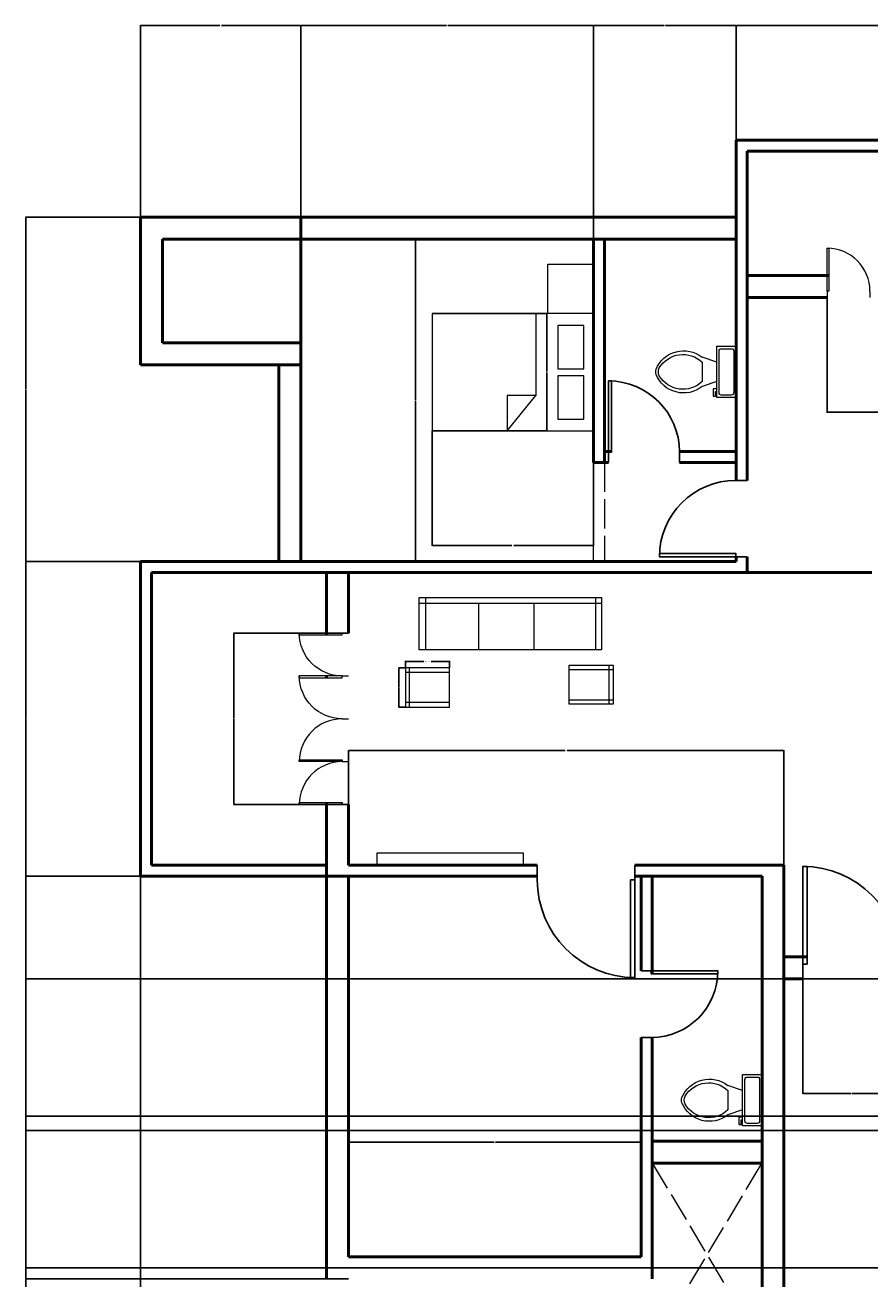
# Model space of a CAD drawing. Units: inches. Extents: x 2032 to 3981, y 840 to 2177.
# Tile 4 of 6: x 2032 to 2378, y 1354 to 1868. Entities that reach past the tile are written whole.
import ezdxf

# ---------------------------------------------------------------- set-up
doc = ezdxf.new("R2010")
doc.units = ezdxf.units.IN
doc.linetypes.add('ACAD_ISO02W100', pattern=[15, 12, -3])
for name, color, linetype, lineweight in [('A-ANNO-DIMS', 2, 'Continuous', 18), ('A-DOOR', 3, 'Continuous', 25), ('A-FLOR-FIXT', 9, 'Continuous', 18), ('A-FLOR-OPEN', 8, 'ACAD_ISO02W100', 13), ('A-FURN', 8, 'Continuous', 18), ('A-GLAZ', 4, 'Continuous', 18), ('A-WALL', 7, 'Continuous', 50), ('A-WALL-OVHD', 8, 'ACAD_ISO02W100', 18)]:
    doc.layers.add(name, color=color, linetype=linetype, lineweight=lineweight)
doc.styles.get("Standard").update_dxf_attribs({"font": 'arial.ttf'})
doc.dimstyles.get("Standard").update_dxf_attribs({"dimtxt": 0.18, "dimasz": 0.18, "dimexe": 0.18, "dimexo": 0.0625, "dimgap": 0.09, "dimtad": 0, "dimtih": 1, "dimtoh": 1, "dimdec": 4, "dimzin": 0, "dimdsep": 46, "dimtxsty": 'Standard', "dimcen": 0.09, "dimadec": 0, "dimazin": 0, "dimtfac": 1, "dimtdec": 4, "dimtofl": 0, "dimtmove": 0, "dimatfit": 3, "dimfxl": 1, "dimtolj": 1, "dimtzin": 0, "dimarcsym": 0})

# ---------------------------------------------------------------- blocks, each defined once
blk = doc.blocks.new('*U2')
for p, q in [((0, 0), (0, -6)), ((40, 0), (40, -6))]:
    blk.add_line(p, q)
blk.add_lwpolyline([(0, 0), (0, 40), (1.75, 40), (1.75, 0)], close=True)
blk.add_arc((0, 0), 40, 0, 90)
blk = doc.blocks.new('*U4')
for p, q in [((9.5, -6), (9.5, -2)), ((-10, -8.5), (-8, -8.5)), ((-10, -9.5), (-10, -8.5)), ((-7, -9.5), (-10, -9.5)), ((-8, -8.5), (-8, -8)), ((-7, -8), (-7, -9.5)), ((-4, -8), (-6, -14)), ((4, -8), (6, -14)), ((4, -14), (-4, -14))]:
    blk.add_line(p, q)
blk.add_lwpolyline([(10.5, -8), (10.5, 0), (-10.5, 0), (-10.5, -8)], close=True)
for points in [[(-9.5, -2), (-9.5, -6)], [(8.5, -1), (-8.5, -1)], [(-8.5, -7), (8.5, -7)]]:
    blk.add_lwpolyline(points)
for centre, radius, start, end in [((-8.62, -1.88), 0.884, 81.8699, 188.1301), ((8.62, -1.88), 0.884, 351.8699, 98.1301), ((-8.62, -6.12), 0.884, 171.8699, 278.1301), ((8.62, -6.12), 0.884, 261.8699, 8.1301), ((3.52, -21.58), 12.17, 141.4691, 247.9714), ((4.2, -21.82), 11.33, 136.3677, 238.9468), ((-3.52, -21.58), 12.17, 292.0284, 38.5307), ((-4.2, -21.82), 11.33, 301.053, 43.6321), ((0, -27.88), 4, 245.7318, 294.2682), ((0, -29), 4, 254.8605, 285.1395)]:
    blk.add_arc(centre, radius, start, end)
blk = doc.blocks.new('CHAIR-LOUNGE')
for p, q in [((1.71, 0), (1.71, 16.03)), ((18.07, 14.22), (0, 14.22)), ((18.07, 1.82), (0, 1.82))]:
    blk.add_line(p, q)
blk.add_lwpolyline([(18.07, 16.03), (0, 16.03), (0, 0), (18.07, 0)], close=True)
blk = doc.blocks.new('*D10')
at = {"layer": 'A-ANNO-DIMS', "color": 0, "lineweight": -2, "transparency": 16777216}
for p, q in [((2187.53, 1604.35), (2187.53, 1607.17)), ((2187.71, 1606.99), (2195.05, 1606.99)), ((2205.43, 1606.99), (2198.09, 1606.99)), ((2205.61, 1604.35), (2205.61, 1607.17))]:
    blk.add_line(p, q, dxfattribs=at)
at = {"layer": 'A-ANNO-DIMS', "color": 0, "lineweight": 100, "transparency": 16777216}
for points in [[(2187.71, 1607.02), (2187.71, 1606.96), (2187.53, 1606.99)], [(2205.43, 1607.02), (2205.43, 1606.96), (2205.61, 1606.99)]]:
    blk.add_solid(points, dxfattribs=at)
at = {"layer": 'Defpoints', "color": 0, "lineweight": 100, "transparency": 16777216}
for p in [(2187.53, 1604.28), (2205.61, 1606.99), (2205.61, 1604.28)]:
    blk.add_point(p, dxfattribs=at)
at = {"layer": 'A-ANNO-DIMS', "color": 0, "transparency": 16777216, "insert": (2196.57, 1606.99), "char_height": 0.18, "attachment_point": 5}
blk.add_mtext('\\A1;LOUNGE CHAIR 18 TYP.', dxfattribs=at)
blk = doc.blocks.new('*D11')
at = {"layer": 'A-ANNO-DIMS', "color": 0, "lineweight": -2, "transparency": 16777216}
for p, q in [((2187.47, 1604.28), (2184.64, 1604.28)), ((2184.82, 1604.1), (2184.82, 1596.45)), ((2184.82, 1588.43), (2184.82, 1596.09)), ((2187.47, 1588.25), (2184.64, 1588.25))]:
    blk.add_line(p, q, dxfattribs=at)
at = {"layer": 'A-ANNO-DIMS', "color": 0, "lineweight": 100, "transparency": 16777216}
for points in [[(2184.79, 1604.1), (2184.85, 1604.1), (2184.82, 1604.28)], [(2184.79, 1588.43), (2184.85, 1588.43), (2184.82, 1588.25)]]:
    blk.add_solid(points, dxfattribs=at)
at = {"layer": 'Defpoints', "color": 0, "lineweight": 100, "transparency": 16777216}
for p in [(2184.82, 1604.28), (2187.53, 1604.28), (2187.53, 1588.25)]:
    blk.add_point(p, dxfattribs=at)
at = {"layer": 'A-ANNO-DIMS', "color": 0, "transparency": 16777216, "insert": (2184.82, 1596.27), "char_height": 0.18, "attachment_point": 5}
blk.add_mtext('\\A1;16 TYP.', dxfattribs=at)
blk = doc.blocks.new('*D14')
at = {"layer": 'A-ANNO-DIMS', "color": 0, "lineweight": -2, "transparency": 16777216}
for p, q in [((2078.89, 1518.9), (2078.89, 840.08)), ((2677.35, 1476.9), (2677.35, 840.08)), ((2079.07, 840.26), (2377.73, 840.26)), ((2677.17, 840.26), (2378.52, 840.26))]:
    blk.add_line(p, q, dxfattribs=at)
at = {"layer": 'A-ANNO-DIMS', "color": 0, "lineweight": 100, "transparency": 16777216}
for points in [[(2079.07, 840.29), (2079.07, 840.23), (2078.89, 840.26)], [(2677.17, 840.29), (2677.17, 840.23), (2677.35, 840.26)]]:
    blk.add_solid(points, dxfattribs=at)
at = {"layer": 'Defpoints', "color": 0, "lineweight": 100, "transparency": 16777216}
for p in [(2078.89, 1518.96), (2677.35, 1476.96), (2677.35, 840.26)]:
    blk.add_point(p, dxfattribs=at)
at = {"layer": 'A-ANNO-DIMS', "color": 0, "transparency": 16777216, "insert": (2378.12, 840.26), "char_height": 0.18, "attachment_point": 5}
blk.add_mtext('\\A1;598.5', dxfattribs=at)
blk = doc.blocks.new('*D16')
at = {"layer": 'A-ANNO-DIMS', "color": 0, "lineweight": -2, "transparency": 16777216}
for p, q in [((2078.89, 1789.02), (2078.89, 1867.7)), ((2079.07, 1867.52), (2111.37, 1867.52)), ((2144.45, 1867.52), (2112.15, 1867.52)), ((2144.63, 1789.02), (2144.63, 1867.7))]:
    blk.add_line(p, q, dxfattribs=at)
at = {"layer": 'A-ANNO-DIMS', "color": 0, "lineweight": 100, "transparency": 16777216}
for points in [[(2079.07, 1867.55), (2079.07, 1867.49), (2078.89, 1867.52)], [(2144.45, 1867.55), (2144.45, 1867.49), (2144.63, 1867.52)]]:
    blk.add_solid(points, dxfattribs=at)
at = {"layer": 'Defpoints', "color": 0, "lineweight": 100, "transparency": 16777216}
for p in [(2144.63, 1867.52), (2078.89, 1788.96), (2144.63, 1788.96)]:
    blk.add_point(p, dxfattribs=at)
at = {"layer": 'A-ANNO-DIMS', "color": 0, "transparency": 16777216, "insert": (2111.76, 1867.52), "char_height": 0.18, "attachment_point": 5}
blk.add_mtext('\\A1;65.74', dxfattribs=at)
blk = doc.blocks.new('*D17')
at = {"layer": 'A-ANNO-DIMS', "color": 0, "lineweight": -2, "transparency": 16777216}
for p, q in [((2144.63, 1789.02), (2144.63, 1867.7)), ((2144.81, 1867.52), (2204.35, 1867.52)), ((2264.45, 1867.52), (2204.91, 1867.52)), ((2264.63, 1780.02), (2264.63, 1867.7))]:
    blk.add_line(p, q, dxfattribs=at)
at = {"layer": 'A-ANNO-DIMS', "color": 0, "lineweight": 100, "transparency": 16777216}
for points in [[(2144.81, 1867.55), (2144.81, 1867.49), (2144.63, 1867.52)], [(2264.45, 1867.55), (2264.45, 1867.49), (2264.63, 1867.52)]]:
    blk.add_solid(points, dxfattribs=at)
at = {"layer": 'Defpoints', "color": 0, "lineweight": 100, "transparency": 16777216}
for p in [(2264.63, 1867.52), (2144.63, 1788.96), (2264.63, 1779.96)]:
    blk.add_point(p, dxfattribs=at)
at = {"layer": 'A-ANNO-DIMS', "color": 0, "transparency": 16777216, "insert": (2204.63, 1867.52), "char_height": 0.18, "attachment_point": 5}
blk.add_mtext('\\A1;120', dxfattribs=at)
blk = doc.blocks.new('*D18')
at = {"layer": 'A-ANNO-DIMS', "color": 0, "lineweight": -2, "transparency": 16777216}
for p, q in [((2264.63, 1780.02), (2264.63, 1867.7)), ((2264.81, 1867.52), (2293.55, 1867.52)), ((2322.95, 1867.52), (2294.2, 1867.52)), ((2323.13, 1820.58), (2323.13, 1867.7))]:
    blk.add_line(p, q, dxfattribs=at)
at = {"layer": 'A-ANNO-DIMS', "color": 0, "lineweight": 100, "transparency": 16777216}
for points in [[(2264.81, 1867.55), (2264.81, 1867.49), (2264.63, 1867.52)], [(2322.95, 1867.55), (2322.95, 1867.49), (2323.13, 1867.52)]]:
    blk.add_solid(points, dxfattribs=at)
at = {"layer": 'Defpoints', "color": 0, "lineweight": 100, "transparency": 16777216}
for p in [(2323.13, 1867.52), (2323.13, 1820.52), (2264.63, 1779.96)]:
    blk.add_point(p, dxfattribs=at)
at = {"layer": 'A-ANNO-DIMS', "color": 0, "transparency": 16777216, "insert": (2293.88, 1867.52), "char_height": 0.18, "attachment_point": 5}
blk.add_mtext('\\A1;58.5', dxfattribs=at)
blk = doc.blocks.new('*D19')
at = {"layer": 'A-ANNO-DIMS', "color": 0, "lineweight": -2, "transparency": 16777216}
for p, q in [((2323.13, 1820.58), (2323.13, 1867.7)), ((2323.31, 1867.52), (2389.49, 1867.52)), ((2456.45, 1867.52), (2390.26, 1867.52)), ((2456.63, 1820.58), (2456.63, 1867.7))]:
    blk.add_line(p, q, dxfattribs=at)
at = {"layer": 'A-ANNO-DIMS', "color": 0, "lineweight": 100, "transparency": 16777216}
for points in [[(2323.31, 1867.55), (2323.31, 1867.49), (2323.13, 1867.52)], [(2456.45, 1867.55), (2456.45, 1867.49), (2456.63, 1867.52)]]:
    blk.add_solid(points, dxfattribs=at)
at = {"layer": 'Defpoints', "color": 0, "lineweight": 100, "transparency": 16777216}
for p in [(2456.63, 1867.52), (2323.13, 1820.52), (2456.63, 1820.52)]:
    blk.add_point(p, dxfattribs=at)
at = {"layer": 'A-ANNO-DIMS', "color": 0, "transparency": 16777216, "insert": (2389.88, 1867.52), "char_height": 0.18, "attachment_point": 5}
blk.add_mtext('\\A1;133.5', dxfattribs=at)
blk = doc.blocks.new('*D24')
at = {"layer": 'A-ANNO-DIMS', "color": 0, "lineweight": -2, "transparency": 16777216}
for p, q in [((2164.15, 1353.96), (2031.71, 1353.96)), ((2031.89, 1353.78), (2031.89, 1276.14)), ((2031.89, 1198.14), (2031.89, 1275.78)), ((2106.03, 1197.96), (2031.71, 1197.96))]:
    blk.add_line(p, q, dxfattribs=at)
at = {"layer": 'A-ANNO-DIMS', "color": 0, "lineweight": 100, "transparency": 16777216}
for points in [[(2031.86, 1353.78), (2031.92, 1353.78), (2031.89, 1353.96)], [(2031.86, 1198.14), (2031.92, 1198.14), (2031.89, 1197.96)]]:
    blk.add_solid(points, dxfattribs=at)
at = {"layer": 'Defpoints', "color": 0, "lineweight": 100, "transparency": 16777216}
for p in [(2031.89, 1353.96), (2164.21, 1353.96), (2106.09, 1197.96)]:
    blk.add_point(p, dxfattribs=at)
at = {"layer": 'A-ANNO-DIMS', "color": 0, "transparency": 16777216, "insert": (2031.89, 1275.96), "char_height": 0.18, "attachment_point": 5}
blk.add_mtext('\\A1;156', dxfattribs=at)
blk = doc.blocks.new('*D25')
at = {"layer": 'A-ANNO-DIMS', "color": 0, "lineweight": -2, "transparency": 16777216}
for p, q in [((2078.83, 1518.96), (2031.71, 1518.96)), ((2031.89, 1518.78), (2031.89, 1436.64)), ((2031.89, 1354.14), (2031.89, 1436.28)), ((2164.15, 1353.96), (2031.71, 1353.96))]:
    blk.add_line(p, q, dxfattribs=at)
at = {"layer": 'A-ANNO-DIMS', "color": 0, "lineweight": 100, "transparency": 16777216}
for points in [[(2031.86, 1518.78), (2031.92, 1518.78), (2031.89, 1518.96)], [(2031.86, 1354.14), (2031.92, 1354.14), (2031.89, 1353.96)]]:
    blk.add_solid(points, dxfattribs=at)
at = {"layer": 'Defpoints', "color": 0, "lineweight": 100, "transparency": 16777216}
for p in [(2031.89, 1518.96), (2078.89, 1518.96), (2164.21, 1353.96)]:
    blk.add_point(p, dxfattribs=at)
at = {"layer": 'A-ANNO-DIMS', "color": 0, "transparency": 16777216, "insert": (2031.89, 1436.46), "char_height": 0.18, "attachment_point": 5}
blk.add_mtext('\\A1;165', dxfattribs=at)
blk = doc.blocks.new('*D26')
at = {"layer": 'A-ANNO-DIMS', "color": 0, "lineweight": -2, "transparency": 16777216}
for p, q in [((2078.83, 1647.96), (2031.71, 1647.96)), ((2031.89, 1647.78), (2031.89, 1583.64)), ((2031.89, 1519.14), (2031.89, 1583.28)), ((2078.83, 1518.96), (2031.71, 1518.96))]:
    blk.add_line(p, q, dxfattribs=at)
at = {"layer": 'A-ANNO-DIMS', "color": 0, "lineweight": 100, "transparency": 16777216}
for points in [[(2031.86, 1647.78), (2031.92, 1647.78), (2031.89, 1647.96)], [(2031.86, 1519.14), (2031.92, 1519.14), (2031.89, 1518.96)]]:
    blk.add_solid(points, dxfattribs=at)
at = {"layer": 'Defpoints', "color": 0, "lineweight": 100, "transparency": 16777216}
for p in [(2031.89, 1647.96), (2078.89, 1647.96), (2078.89, 1518.96)]:
    blk.add_point(p, dxfattribs=at)
at = {"layer": 'A-ANNO-DIMS', "color": 0, "transparency": 16777216, "insert": (2031.89, 1583.46), "char_height": 0.18, "attachment_point": 5}
blk.add_mtext('\\A1;129', dxfattribs=at)
blk = doc.blocks.new('*D27')
at = {"layer": 'A-ANNO-DIMS', "color": 0, "lineweight": -2, "transparency": 16777216}
for p, q in [((2078.83, 1788.96), (2031.71, 1788.96)), ((2031.89, 1788.78), (2031.89, 1718.64)), ((2031.89, 1648.14), (2031.89, 1718.28)), ((2078.83, 1647.96), (2031.71, 1647.96))]:
    blk.add_line(p, q, dxfattribs=at)
at = {"layer": 'A-ANNO-DIMS', "color": 0, "lineweight": 100, "transparency": 16777216}
for points in [[(2031.86, 1788.78), (2031.92, 1788.78), (2031.89, 1788.96)], [(2031.86, 1648.14), (2031.92, 1648.14), (2031.89, 1647.96)]]:
    blk.add_solid(points, dxfattribs=at)
at = {"layer": 'Defpoints', "color": 0, "lineweight": 100, "transparency": 16777216}
for p in [(2031.89, 1788.96), (2078.89, 1788.96), (2078.89, 1647.96)]:
    blk.add_point(p, dxfattribs=at)
at = {"layer": 'A-ANNO-DIMS', "color": 0, "transparency": 16777216, "insert": (2031.89, 1718.46), "char_height": 0.18, "attachment_point": 5}
blk.add_mtext('\\A1;141', dxfattribs=at)
blk = doc.blocks.new('*D28')
at = {"layer": 'A-ANNO-DIMS', "color": 0, "lineweight": -2, "transparency": 16777216}
for p, q in [((2144.69, 1779.96), (2191.81, 1779.96)), ((2191.63, 1779.78), (2191.63, 1714.14)), ((2191.63, 1648.14), (2191.63, 1713.78)), ((2144.69, 1647.96), (2191.81, 1647.96))]:
    blk.add_line(p, q, dxfattribs=at)
at = {"layer": 'A-ANNO-DIMS', "color": 0, "lineweight": 100, "transparency": 16777216}
for points in [[(2191.6, 1779.78), (2191.66, 1779.78), (2191.63, 1779.96)], [(2191.6, 1648.14), (2191.66, 1648.14), (2191.63, 1647.96)]]:
    blk.add_solid(points, dxfattribs=at)
at = {"layer": 'Defpoints', "color": 0, "lineweight": 100, "transparency": 16777216}
for p in [(2144.63, 1779.96), (2144.63, 1647.96), (2191.63, 1647.96)]:
    blk.add_point(p, dxfattribs=at)
at = {"layer": 'A-ANNO-DIMS', "color": 0, "transparency": 16777216, "insert": (2191.63, 1713.96), "char_height": 0.18, "attachment_point": 5}
blk.add_mtext('\\A1;132', dxfattribs=at)
blk = doc.blocks.new('*D29')
at = {"layer": 'A-ANNO-DIMS', "color": 0, "lineweight": -2, "transparency": 16777216}
for p, q in [((2198.45, 1701.44), (2198.45, 1654.32)), ((2264.63, 1701.44), (2264.63, 1654.32)), ((2198.63, 1654.5), (2231.14, 1654.5)), ((2264.45, 1654.5), (2231.93, 1654.5))]:
    blk.add_line(p, q, dxfattribs=at)
at = {"layer": 'A-ANNO-DIMS', "color": 0, "lineweight": 100, "transparency": 16777216}
for points in [[(2198.63, 1654.53), (2198.63, 1654.47), (2198.45, 1654.5)], [(2264.45, 1654.53), (2264.45, 1654.47), (2264.63, 1654.5)]]:
    blk.add_solid(points, dxfattribs=at)
at = {"layer": 'Defpoints', "color": 0, "lineweight": 100, "transparency": 16777216}
for p in [(2198.45, 1701.5), (2264.63, 1701.5), (2198.45, 1654.5)]:
    blk.add_point(p, dxfattribs=at)
at = {"layer": 'A-ANNO-DIMS', "color": 0, "transparency": 16777216, "insert": (2231.54, 1654.5), "char_height": 0.18, "attachment_point": 5}
blk.add_mtext('\\A1;66.18', dxfattribs=at)
blk = doc.blocks.new('*D30')
at = {"layer": 'A-ANNO-DIMS', "color": 0, "lineweight": -2, "transparency": 16777216}
for p, q in [((2198.51, 1749.53), (2245.63, 1749.53)), ((2245.45, 1749.35), (2245.45, 1725.7)), ((2245.45, 1701.68), (2245.45, 1725.33)), ((2198.51, 1701.5), (2245.63, 1701.5))]:
    blk.add_line(p, q, dxfattribs=at)
at = {"layer": 'A-ANNO-DIMS', "color": 0, "lineweight": 100, "transparency": 16777216}
for points in [[(2245.42, 1749.35), (2245.48, 1749.35), (2245.45, 1749.53)], [(2245.42, 1701.68), (2245.48, 1701.68), (2245.45, 1701.5)]]:
    blk.add_solid(points, dxfattribs=at)
at = {"layer": 'Defpoints', "color": 0, "lineweight": 100, "transparency": 16777216}
for p in [(2198.45, 1749.53), (2198.45, 1701.5), (2245.45, 1701.5)]:
    blk.add_point(p, dxfattribs=at)
at = {"layer": 'A-ANNO-DIMS', "color": 0, "transparency": 16777216, "insert": (2245.45, 1725.52), "char_height": 0.18, "attachment_point": 5}
blk.add_mtext('\\A1;48.03', dxfattribs=at)
blk = doc.blocks.new('*D32')
at = {"layer": 'A-ANNO-DIMS', "color": 0, "lineweight": -2, "transparency": 16777216}
for p, q in [((2360.39, 1756), (2360.39, 1708.89)), ((2430.64, 1756), (2430.64, 1708.89)), ((2360.57, 1709.07), (2395.12, 1709.07)), ((2430.46, 1709.07), (2395.91, 1709.07))]:
    blk.add_line(p, q, dxfattribs=at)
at = {"layer": 'A-ANNO-DIMS', "color": 0, "lineweight": 100, "transparency": 16777216}
for points in [[(2360.57, 1709.1), (2360.57, 1709.04), (2360.39, 1709.07)], [(2430.46, 1709.1), (2430.46, 1709.04), (2430.64, 1709.07)]]:
    blk.add_solid(points, dxfattribs=at)
at = {"layer": 'Defpoints', "color": 0, "lineweight": 100, "transparency": 16777216}
for p in [(2360.39, 1756.07), (2430.64, 1756.07), (2360.39, 1709.07)]:
    blk.add_point(p, dxfattribs=at)
at = {"layer": 'A-ANNO-DIMS', "color": 0, "transparency": 16777216, "insert": (2395.51, 1709.07), "char_height": 0.18, "attachment_point": 5}
blk.add_mtext('\\A1;70.24', dxfattribs=at)
blk = doc.blocks.new('*D33')
at = {"layer": 'A-ANNO-DIMS', "color": 0, "lineweight": -2, "transparency": 16777216}
for p, q in [((2164.21, 1523.52), (2164.21, 1570.64)), ((2164.39, 1570.46), (2253.07, 1570.46)), ((2342.53, 1570.46), (2253.85, 1570.46)), ((2342.71, 1523.52), (2342.71, 1570.64))]:
    blk.add_line(p, q, dxfattribs=at)
at = {"layer": 'A-ANNO-DIMS', "color": 0, "lineweight": 100, "transparency": 16777216}
for points in [[(2164.39, 1570.49), (2164.39, 1570.43), (2164.21, 1570.46)], [(2342.53, 1570.49), (2342.53, 1570.43), (2342.71, 1570.46)]]:
    blk.add_solid(points, dxfattribs=at)
at = {"layer": 'Defpoints', "color": 0, "lineweight": 100, "transparency": 16777216}
for p in [(2342.71, 1570.46), (2164.21, 1523.46), (2342.71, 1523.46)]:
    blk.add_point(p, dxfattribs=at)
at = {"layer": 'A-ANNO-DIMS', "color": 0, "transparency": 16777216, "insert": (2253.46, 1570.46), "char_height": 0.18, "attachment_point": 5}
blk.add_mtext('\\A1;178.5', dxfattribs=at)
blk = doc.blocks.new('*D34')
at = {"layer": 'A-ANNO-DIMS', "color": 0, "lineweight": -2, "transparency": 16777216}
for p, q in [((2164.15, 1618.58), (2117.03, 1618.58)), ((2117.21, 1618.4), (2117.21, 1583.64)), ((2117.21, 1548.52), (2117.21, 1583.28)), ((2164.15, 1548.34), (2117.03, 1548.34))]:
    blk.add_line(p, q, dxfattribs=at)
at = {"layer": 'A-ANNO-DIMS', "color": 0, "lineweight": 100, "transparency": 16777216}
for points in [[(2117.18, 1618.4), (2117.24, 1618.4), (2117.21, 1618.58)], [(2117.18, 1548.52), (2117.24, 1548.52), (2117.21, 1548.34)]]:
    blk.add_solid(points, dxfattribs=at)
at = {"layer": 'Defpoints', "color": 0, "lineweight": 100, "transparency": 16777216}
for p in [(2117.21, 1618.58), (2164.21, 1618.58), (2164.21, 1548.34)]:
    blk.add_point(p, dxfattribs=at)
at = {"layer": 'A-ANNO-DIMS', "color": 0, "transparency": 16777216, "insert": (2117.21, 1583.46), "char_height": 0.18, "attachment_point": 5}
blk.add_mtext('\\A1;70.24', dxfattribs=at)
blk = doc.blocks.new('*D37')
at = {"layer": 'A-ANNO-DIMS', "color": 0, "lineweight": -2, "transparency": 16777216}
for p, q in [((2350.44, 1476.9), (2350.44, 1429.78)), ((2390.44, 1476.9), (2390.44, 1429.78)), ((2350.62, 1429.96), (2370.22, 1429.96)), ((2390.26, 1429.96), (2370.66, 1429.96))]:
    blk.add_line(p, q, dxfattribs=at)
at = {"layer": 'A-ANNO-DIMS', "color": 0, "lineweight": 100, "transparency": 16777216}
for points in [[(2350.62, 1429.99), (2350.62, 1429.93), (2350.44, 1429.96)], [(2390.26, 1429.99), (2390.26, 1429.93), (2390.44, 1429.96)]]:
    blk.add_solid(points, dxfattribs=at)
at = {"layer": 'Defpoints', "color": 0, "lineweight": 100, "transparency": 16777216}
for p in [(2350.44, 1476.96), (2390.44, 1476.96), (2350.44, 1429.96)]:
    blk.add_point(p, dxfattribs=at)
at = {"layer": 'A-ANNO-DIMS', "color": 0, "transparency": 16777216, "insert": (2370.44, 1429.96), "char_height": 0.18, "attachment_point": 5}
blk.add_mtext('\\A1;40', dxfattribs=at)
blk = doc.blocks.new('*D38')
at = {"layer": 'A-ANNO-DIMS', "color": 0, "lineweight": -2, "transparency": 16777216}
for p, q in [((2164.21, 1363.02), (2164.21, 1410.14)), ((2164.39, 1409.96), (2223.93, 1409.96)), ((2284.03, 1409.96), (2224.49, 1409.96)), ((2284.21, 1363.02), (2284.21, 1410.14))]:
    blk.add_line(p, q, dxfattribs=at)
at = {"layer": 'A-ANNO-DIMS', "color": 0, "lineweight": 100, "transparency": 16777216}
for points in [[(2164.39, 1409.99), (2164.39, 1409.93), (2164.21, 1409.96)], [(2284.03, 1409.99), (2284.03, 1409.93), (2284.21, 1409.96)]]:
    blk.add_solid(points, dxfattribs=at)
at = {"layer": 'Defpoints', "color": 0, "lineweight": 100, "transparency": 16777216}
for p in [(2284.21, 1409.96), (2164.21, 1362.96), (2284.21, 1362.96)]:
    blk.add_point(p, dxfattribs=at)
at = {"layer": 'A-ANNO-DIMS', "color": 0, "transparency": 16777216, "insert": (2224.21, 1409.96), "char_height": 0.18, "attachment_point": 5}
blk.add_mtext('\\A1;120', dxfattribs=at)
blk = doc.blocks.new('*D66')
at = {"layer": 'A-ANNO-DIMS', "color": 0, "lineweight": -2, "transparency": 16777216}
for p, q in [((2461.87, 1414.71), (2031.71, 1414.71)), ((2031.89, 1414.53), (2031.89, 1386.77)), ((2031.89, 1358.64), (2031.89, 1386.4)), ((2461.87, 1358.46), (2031.71, 1358.46))]:
    blk.add_line(p, q, dxfattribs=at)
at = {"layer": 'A-ANNO-DIMS', "color": 0, "lineweight": 100, "transparency": 16777216}
for points in [[(2031.86, 1414.53), (2031.92, 1414.53), (2031.89, 1414.71)], [(2031.86, 1358.64), (2031.92, 1358.64), (2031.89, 1358.46)]]:
    blk.add_solid(points, dxfattribs=at)
at = {"layer": 'Defpoints', "color": 0, "lineweight": 100, "transparency": 16777216}
for p in [(2461.93, 1414.71), (2031.89, 1358.46), (2461.93, 1358.46)]:
    blk.add_point(p, dxfattribs=at)
at = {"layer": 'A-ANNO-DIMS', "color": 0, "transparency": 16777216, "insert": (2031.89, 1386.58), "char_height": 0.18, "attachment_point": 5}
blk.add_mtext('\\A1;56.25', dxfattribs=at)
blk = doc.blocks.new('*D67')
at = {"layer": 'A-ANNO-DIMS', "color": 0, "lineweight": -2, "transparency": 16777216}
for p, q in [((2461.87, 1476.96), (2031.71, 1476.96)), ((2031.89, 1476.78), (2031.89, 1449.02)), ((2031.89, 1420.89), (2031.89, 1448.65)), ((2461.87, 1420.71), (2031.71, 1420.71))]:
    blk.add_line(p, q, dxfattribs=at)
at = {"layer": 'A-ANNO-DIMS', "color": 0, "lineweight": 100, "transparency": 16777216}
for points in [[(2031.86, 1476.78), (2031.92, 1476.78), (2031.89, 1476.96)], [(2031.86, 1420.89), (2031.92, 1420.89), (2031.89, 1420.71)]]:
    blk.add_solid(points, dxfattribs=at)
at = {"layer": 'Defpoints', "color": 0, "lineweight": 100, "transparency": 16777216}
for p in [(2461.93, 1476.96), (2031.89, 1420.71), (2461.93, 1420.71)]:
    blk.add_point(p, dxfattribs=at)
at = {"layer": 'A-ANNO-DIMS', "color": 0, "transparency": 16777216, "insert": (2031.89, 1448.83), "char_height": 0.18, "attachment_point": 5}
blk.add_mtext('\\A1;56.25', dxfattribs=at)

msp = doc.modelspace()

# ---------------------------------------------------------------- linework, layer by layer
at = {"layer": 'A-FLOR-OPEN'}
for p, q in [((2288.7092, 1326.1705), (2333.7092, 1401.441)), ((2288.7092, 1401.441), (2333.7092, 1326.1705))]:
    msp.add_line(p, q, dxfattribs=at)
at = {"layer": 'A-FURN'}
for p, q in [((2240.9244, 1749.5297), (2240.9244, 1715.8749)), ((2240.9244, 1715.8749), (2229.239, 1715.8749)), ((2229.239, 1715.8749), (2229.239, 1701.5024)), ((2229.239, 1701.5024), (2240.9244, 1715.8749)), ((2193.1759, 1630.849), (2267.8949, 1630.849)), ((2195.8972, 1611.689), (2195.8972, 1633.1846)), ((2217.4159, 1630.849), (2217.4159, 1611.689)), ((2240.1936, 1630.849), (2240.1936, 1611.689)), ((2265.604, 1611.689), (2265.604, 1633.1846))]:
    msp.add_line(p, q, dxfattribs=at)
for points in [[(2264.6278, 1749.5297), (2245.9514, 1749.5297), (2245.9514, 1769.7069), (2264.6278, 1769.7069)], [(2264.6278, 1749.5297), (2198.4509, 1749.5297), (2198.4509, 1701.5024), (2264.6278, 1701.5024)], [(2260.6872, 1744.6198), (2250.0491, 1744.6198), (2250.0491, 1726.8305), (2260.6872, 1726.8305)], [(2260.6872, 1723.9775), (2250.0491, 1723.9775), (2250.0491, 1706.1882), (2260.6872, 1706.1882)], [(2193.1759, 1633.1846), (2267.8949, 1633.1846), (2267.8949, 1611.689), (2193.1759, 1611.689)], [(2235.7903, 1523.4584), (2175.8891, 1523.4584), (2175.8891, 1528.5804), (2235.7903, 1528.5804)]]:
    msp.add_lwpolyline(points, close=True, dxfattribs=at)
at = {"layer": 'A-WALL'}
for p, q in [((2323.1278, 1779.9584), (2323.1278, 1820.5217)), ((2323.1278, 1820.5217), (2456.6278, 1820.5217)), ((2327.6278, 1779.9584), (2327.6278, 1816.0217)), ((2327.6278, 1816.0217), (2452.1278, 1816.0217)), ((2135.6278, 1788.9584), (2078.8911, 1788.9584)), ((2078.8911, 1788.9584), (2078.8911, 1728.4681)), ((2135.6278, 1788.9584), (2323.1278, 1788.9584)), ((2144.6278, 1779.9584), (2144.6278, 1788.9584)), ((2144.6278, 1788.9584), (2144.6278, 1779.9584)), ((2135.6278, 1779.9584), (2087.8911, 1779.9584)), ((2087.8911, 1779.9584), (2087.8911, 1737.4681)), ((2144.6278, 1779.9584), (2135.6278, 1779.9584)), ((2144.6278, 1779.9584), (2264.6278, 1779.9584)), ((2144.6278, 1647.9584), (2144.6278, 1779.9584)), ((2264.6278, 1779.9584), (2264.6278, 1688.4584)), ((2264.6278, 1779.9584), (2269.1278, 1779.9584)), ((2269.1278, 1779.9584), (2269.1278, 1688.4584)), ((2269.1278, 1779.9584), (2323.1278, 1779.9584)), ((2323.1278, 1779.9584), (2323.1278, 1692.9584)), ((2327.6278, 1779.9584), (2327.6278, 1688.4584)), ((2327.6278, 1765.0659), (2361.1603, 1765.0659)), ((2327.6278, 1756.0659), (2360.392, 1756.0659)), ((2087.8911, 1737.4681), (2144.6278, 1737.4681)), ((2078.8911, 1728.4681), (2144.6278, 1728.4681)), ((2135.6278, 1647.9584), (2135.6278, 1728.4681)), ((2272.0483, 1692.9584), (2269.1278, 1692.9584)), ((2323.1278, 1692.9584), (2299.8623, 1692.9584)), ((2323.1278, 1692.9584), (2323.1278, 1681.1427)), ((2269.1278, 1688.4584), (2264.6278, 1688.4584)), ((2270.7758, 1688.4584), (2269.1278, 1688.4584)), ((2323.1278, 1688.4584), (2299.8627, 1688.4584)), ((2327.6278, 1688.4584), (2327.6278, 1681.1427)), ((2323.1278, 1649.849), (2323.1278, 1647.9584)), ((2327.6278, 1649.849), (2327.6278, 1643.4584)), ((2078.8911, 1518.9584), (2078.8911, 1647.9584)), ((2078.8911, 1647.9584), (2144.6278, 1647.9584)), ((2264.6278, 1647.9584), (2144.6278, 1647.9584)), ((2264.6278, 1647.9584), (2269.1278, 1647.9584)), ((2269.1278, 1647.9584), (2323.1278, 1647.9584)), ((2083.3911, 1523.4584), (2083.3911, 1643.4584)), ((2083.3911, 1643.4584), (2144.6278, 1643.4584)), ((2269.1278, 1643.4584), (2135.6278, 1643.4584)), ((2155.2092, 1643.4584), (2155.2092, 1617.8118)), ((2164.2092, 1643.4584), (2164.2092, 1618.58)), ((2378.7092, 1643.4584), (2269.1278, 1643.4584)), ((2155.2092, 1601.0192), (2155.2092, 1600.2509)), ((2155.2092, 1566.6659), (2155.2092, 1565.8976)), ((2155.2092, 1549.1051), (2155.2092, 1518.9584)), ((2164.2092, 1548.3368), (2164.2092, 1523.4584)), ((2155.2092, 1523.4584), (2083.3911, 1523.4584)), ((2164.2092, 1523.4584), (2241.5909, 1523.4584)), ((2281.5909, 1523.4584), (2342.7092, 1523.4584)), ((2342.7092, 1518.9584), (2342.7092, 1523.4584)), ((2155.2092, 1518.9584), (2078.8911, 1518.9584)), ((2155.2092, 1518.9584), (2241.5909, 1518.9584)), ((2155.2092, 1518.9584), (2155.2092, 1353.9584)), ((2164.2092, 1518.9584), (2164.2092, 1362.9584)), ((2281.5909, 1518.9584), (2333.7092, 1518.9584)), ((2284.2092, 1480.1774), (2284.2092, 1518.9584)), ((2288.7092, 1478.9826), (2288.7092, 1518.9584)), ((2333.7092, 1293.9584), (2333.7092, 1518.9584)), ((2342.7092, 1302.9584), (2342.7092, 1518.9584)), ((2352.1882, 1485.9584), (2342.7092, 1485.9584)), ((2350.4382, 1476.9584), (2342.7092, 1476.9584)), ((2284.2092, 1362.9584), (2284.2092, 1452.8679)), ((2288.7092, 1353.9584), (2288.7092, 1452.8709)), ((2288.7092, 1410.441), (2333.7092, 1410.441)), ((2288.7092, 1401.441), (2333.7092, 1401.441)), ((2164.2092, 1362.9584), (2284.2092, 1362.9584))]:
    msp.add_line(p, q, dxfattribs=at)
at = {"layer": 'A-WALL-OVHD'}
msp.add_lwpolyline([(2264.6278, 1688.4584), (2269.1278, 1688.4584), (2269.1278, 1647.9584), (2264.6278, 1647.9584)], close=True, dxfattribs=at)

# ---------------------------------------------------------------- block references
at = {"layer": 'A-DOOR', "xscale": 0.7271725307901341, "yscale": 0.7271725307901341, "zscale": 0.7271725307901341}
msp.add_blockref('*U2', (2270.7758, 1692.8215), dxfattribs=at)
at = {"layer": 'A-DOOR'}
for p, xscale, yscale, zscale, rotation in [((2322.9337, 1649.849), 0.7823425013316796, 0.7823425013316796, 0.7823425013316796, 90), ((2288.3056, 1480.1774), 0.6827360457483597, 0.6827360457483597, 0.6827360457483597, 270)]:
    msp.add_blockref('*U2', p, dxfattribs=dict(at, xscale=xscale, yscale=yscale, zscale=zscale, rotation=rotation))
at = {"layer": 'A-DOOR', "rotation": 180}
msp.add_blockref('*U2', (2281.5909, 1517.4584), dxfattribs=at)
at = {"layer": 'A-DOOR'}
msp.add_blockref('*U2', (2350.4382, 1482.9584), dxfattribs=at)
at = {"layer": 'A-FLOR-FIXT', "xscale": -1, "rotation": 270}
for p in [(2323.1278, 1725.6125), (2333.7092, 1427.1878)]:
    msp.add_blockref('*U4', p, dxfattribs=at)
at = {"layer": 'A-FURN'}
msp.add_blockref('CHAIR-LOUNGE', (2187.533, 1588.251), dxfattribs=at)
at = {"layer": 'A-FURN', "extrusion": (0, 0, -1), "zscale": -1}
msp.add_blockref('CHAIR-LOUNGE', (-2272.7413, 1589.4415), dxfattribs=at)
at = {"layer": 'A-GLAZ', "xscale": 0.4390204122695697, "yscale": 0.4390204122695697, "zscale": 0.4390204122695697}
msp.add_blockref('*U2', (2360.392, 1758.7001), dxfattribs=at)
at = {"layer": 'A-GLAZ', "yscale": 0.4390204122695697, "zscale": 0.4390204122695697, "rotation": 90}
for p, xscale in [((2161.5751, 1618.58), -0.4390204122695697), ((2161.5751, 1601.0192), -0.4390204122695697), ((2161.5751, 1565.8976), 0.4390204122695697), ((2161.5751, 1548.3368), 0.4390204122695697)]:
    msp.add_blockref('*U2', p, dxfattribs=dict(at, xscale=xscale))

# ---------------------------------------------------------------- dimensions: what is measured, and where the dimension line sits
at = {"layer": 'A-ANNO-DIMS'}
for base, p1, p2, override, picture, middle in [((2144.6278, 1867.5217), (2078.8911, 1788.9584), (2144.6278, 1788.9584), {"dimdec": 2, "dimlfac": 1, "dimrnd": 0, "dimzin": 0, "dimdsep": 46, "dimlunit": 2}, '*D16', (2111.7595, 1867.5217)), ((2264.6278, 1867.5217), (2144.6278, 1788.9584), (2264.6278, 1779.9584), {"dimdec": 0, "dimlfac": 1, "dimrnd": 0, "dimzin": 0, "dimdsep": 46, "dimlunit": 2}, '*D17', (2204.6278, 1867.5217)), ((2323.1278, 1867.5217), (2264.6278, 1779.9584), (2323.1278, 1820.5217), {"dimdec": 1, "dimlfac": 1, "dimrnd": 0, "dimzin": 0, "dimdsep": 46, "dimlunit": 2}, '*D18', (2293.8778, 1867.5217)), ((2456.6278, 1867.5217), (2323.1278, 1820.5217), (2456.6278, 1820.5217), {"dimdec": 1, "dimlfac": 1, "dimrnd": 0, "dimzin": 0, "dimdsep": 46, "dimlunit": 2}, '*D19', (2389.8778, 1867.5217)), ((2342.7092, 1570.4584), (2164.2092, 1523.4584), (2342.7092, 1523.4584), {"dimdec": 1, "dimlfac": 1, "dimrnd": 0, "dimzin": 0, "dimdsep": 46, "dimlunit": 2}, '*D33', (2253.4592, 1570.4584)), ((2677.3537, 840.2551), (2078.8911, 1518.9584), (2677.3537, 1476.9584), {"dimdec": 1, "dimlfac": 1, "dimrnd": 0, "dimzin": 0, "dimdsep": 46, "dimlunit": 2}, '*D14', (2378.1224, 840.2551)), ((2284.2092, 1409.9584), (2164.2092, 1362.9584), (2284.2092, 1362.9584), {"dimdec": 0, "dimlfac": 1, "dimrnd": 0, "dimzin": 0, "dimdsep": 46, "dimlunit": 2}, '*D38', (2224.2092, 1409.9584))]:
    dim = msp.add_linear_dim(base=base, p1=p1, p2=p2, dimstyle='Standard', override=override, dxfattribs=at)
    dim.commit()
    dim.dimension.update_dxf_attribs({"geometry": picture, "text_midpoint": middle})
for base, p1, p2, angle, override, picture, middle in [((2031.8911, 1788.9584), (2078.8911, 1647.9584), (2078.8911, 1788.9584), 90, {"dimdec": 0, "dimlfac": 1, "dimrnd": 0, "dimzin": 0, "dimdsep": 46, "dimlunit": 2}, '*D27', (2031.8911, 1718.4584)), ((2191.6278, 1647.9584), (2144.6278, 1779.9584), (2144.6278, 1647.9584), 270, {"dimdec": 0, "dimlfac": 1, "dimrnd": 0, "dimzin": 0, "dimdsep": 46, "dimlunit": 2}, '*D28', (2191.6278, 1713.9584)), ((2360.392, 1709.0659), (2430.6353, 1756.0659), (2360.392, 1756.0659), 180, {"dimdec": 2, "dimlfac": 1, "dimrnd": 0, "dimzin": 0, "dimdsep": 46, "dimlunit": 2}, '*D32', (2395.5137, 1709.0659)), ((2245.4509, 1701.5024), (2198.4509, 1749.5297), (2198.4509, 1701.5024), 270, {"dimdec": 2, "dimlfac": 1, "dimrnd": 0, "dimzin": 0, "dimdsep": 46, "dimlunit": 2}, '*D30', (2245.4509, 1725.516)), ((2198.4509, 1654.5024), (2264.6278, 1701.5024), (2198.4509, 1701.5024), 180, {"dimdec": 2, "dimlfac": 1, "dimrnd": 0, "dimzin": 0, "dimdsep": 46, "dimlunit": 2}, '*D29', (2231.5393, 1654.5024)), ((2031.8911, 1647.9584), (2078.8911, 1518.9584), (2078.8911, 1647.9584), 90, {"dimdec": 0, "dimlfac": 1, "dimrnd": 0, "dimzin": 0, "dimdsep": 46, "dimlunit": 2}, '*D26', (2031.8911, 1583.4584)), ((2117.2092, 1618.58), (2164.2092, 1548.3368), (2164.2092, 1618.58), 90, {"dimdec": 2, "dimlfac": 1, "dimrnd": 0, "dimzin": 0, "dimdsep": 46, "dimlunit": 2}, '*D34', (2117.2092, 1583.4584)), ((2031.8911, 1518.9584), (2164.2092, 1353.9584), (2078.8911, 1518.9584), 90, {"dimdec": 0, "dimlfac": 1, "dimrnd": 0, "dimzin": 0, "dimdsep": 46, "dimlunit": 2}, '*D25', (2031.8911, 1436.4584)), ((2031.8911, 1420.7084), (2461.9346, 1476.9584), (2461.9346, 1420.7084), 90, {"dimdec": 2, "dimlfac": 1, "dimrnd": 0, "dimzin": 0, "dimdsep": 46, "dimlunit": 2}, '*D67', (2031.8911, 1448.8334)), ((2350.4382, 1429.9584), (2390.4382, 1476.9584), (2350.4382, 1476.9584), 180, {"dimdec": 0, "dimlfac": 1, "dimrnd": 0, "dimzin": 0, "dimdsep": 46, "dimlunit": 2}, '*D37', (2370.4382, 1429.9584)), ((2031.8911, 1358.4584), (2461.9346, 1414.7084), (2461.9346, 1358.4584), 90, {"dimdec": 2, "dimlfac": 1, "dimrnd": 0, "dimzin": 0, "dimdsep": 46, "dimlunit": 2}, '*D66', (2031.8911, 1386.5834)), ((2031.8911, 1353.9584), (2106.0893, 1197.9584), (2164.2092, 1353.9584), 90, {"dimdec": 0, "dimlfac": 1, "dimrnd": 0, "dimzin": 0, "dimdsep": 46, "dimlunit": 2}, '*D24', (2031.8911, 1275.9584))]:
    dim = msp.add_linear_dim(base=base, p1=p1, p2=p2, angle=angle, dimstyle='Standard', override=override, dxfattribs=at)
    dim.commit()
    dim.dimension.update_dxf_attribs({"geometry": picture, "text_midpoint": middle})
dim = msp.add_linear_dim(base=(2184.8223, 1604.2828), p1=(2187.5335, 1588.2513), p2=(2187.5335, 1604.2828), angle=90, text='<> TYP.', dimstyle='Standard', override={"dimdec": 0, "dimlfac": 1, "dimrnd": 0, "dimzin": 0, "dimdsep": 46, "dimlunit": 2}, dxfattribs=at)
dim.commit()
dim.dimension.update_dxf_attribs({"geometry": '*D11', "text_midpoint": (2184.8223, 1596.267)})
dim = msp.add_linear_dim(base=(2205.6078, 1606.9939), p1=(2187.5335, 1604.2828), p2=(2205.6078, 1604.2828), text='LOUNGE CHAIR <> TYP.', dimstyle='Standard', override={"dimdec": 0, "dimlfac": 1, "dimrnd": 0, "dimzin": 0, "dimdsep": 46, "dimlunit": 2}, dxfattribs=at)
dim.commit()
dim.dimension.update_dxf_attribs({"geometry": '*D10', "text_midpoint": (2196.5706, 1606.9939)})

doc.saveas('drawing.dxf')
